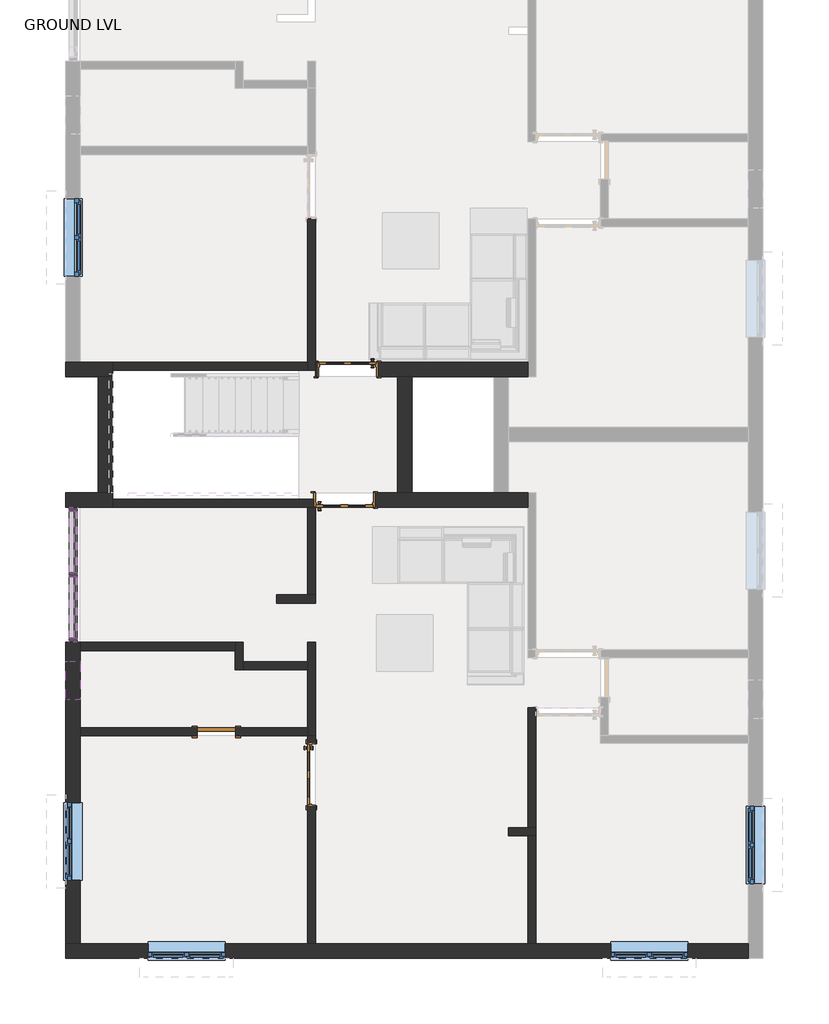
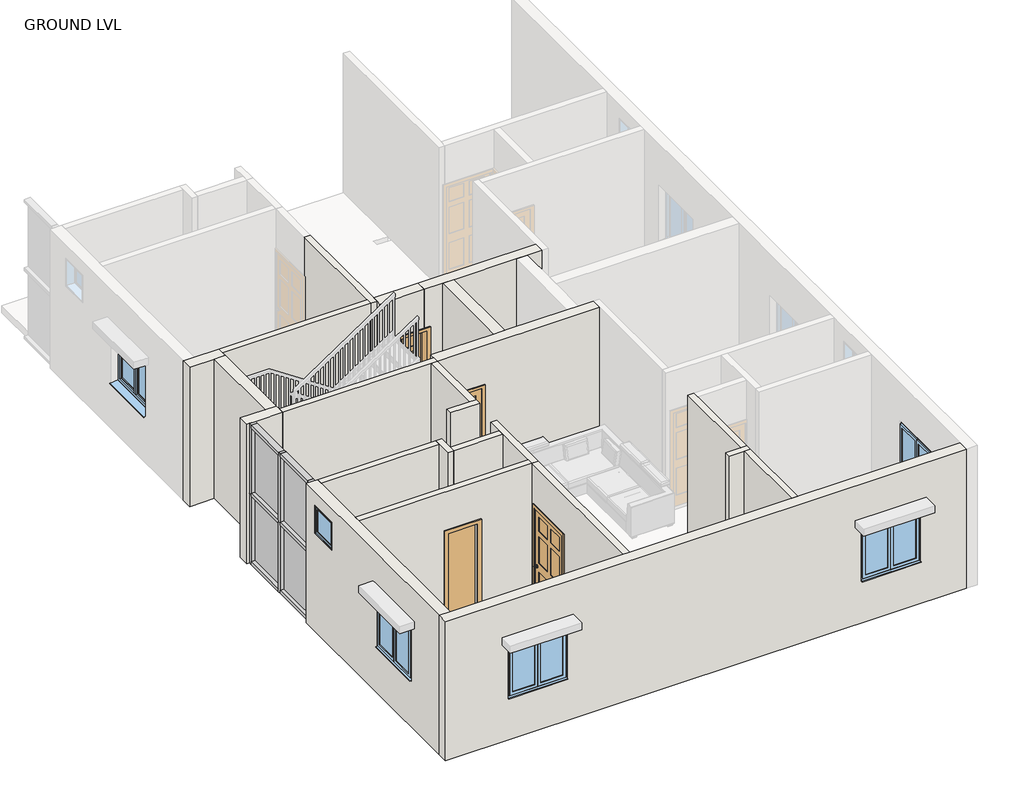
# One storey, part 1 of 4: 23 walls, 12 members, 6 windows, 4 doors, 4 plates.
"""IFC4 building model written with IfcOpenShell, lengths in millimetres."""

from ifc_helpers import new_model, si_unit, frame, origin, place, context, project, spatial, polyline, outline, extrude, faceted_brep, transform, mapped, element, save
from components import door_6a452240, door_interior_single_6_panel_wood_interior_door_3_x_7_c5239341, single_flush_flush_door_2_x_7_931cabab, member_801a2072, member_82905deb, member_88aa5c81, member_4491d118, system_panel_glazed_a8655be6, window_80340324, w2_windows_4_x_4_9dec5fc7

model = new_model("IFC4")

# Units and contexts
model_context = context("Model", 3, world=origin())
ifc_project = project(units=[si_unit("LENGTHUNIT", "METRE", prefix="MILLI")], contexts=[model_context])

# Site, building, storey
site = spatial("IfcSite", under=ifc_project)
building = spatial("IfcBuilding", under=site)
storey = spatial("IfcBuildingStorey", under=building, Name="GROUND LVL", Elevation=3048.0)

# Doors
placement = place(None, origin())
door_shape = door_6a452240(model_context)
element("IfcDoor", 1, ObjectType="Door-Interior-Single-6_Panel-Wood : interior door 3' 4\" x 7'", at=placement, inside=storey, context=model_context, shape_type="MappedRepresentation", body=[
    mapped(door_shape, transform((-2560.6762202, -343.1690997, 3048.0), x_axis=(0.0, -1.0, 0.0), y_axis=(1.0, 0.0, 0.0), z_axis=(0.0, 0.0, 1.0))),
])
door_interior_single_6_panel_wood_interior_door_3_x_7_shape = door_interior_single_6_panel_wood_interior_door_3_x_7_c5239341(model_context)
element("IfcDoor", 2, ObjectType="Door-Interior-Single-6_Panel-Wood : interior door 3' x 7'", at=placement, inside=storey, context=model_context, shape_type="MappedRepresentation", body=[
    mapped(door_interior_single_6_panel_wood_interior_door_3_x_7_shape, transform((-1986.0012202, 6048.1059003, 3048.0), x_axis=(-1.0, 0.0, 0.0), y_axis=(0.0, -1.0, 0.0), z_axis=(0.0, 0.0, 1.0))),
])
element("IfcDoor", 3, ObjectType="Door-Interior-Single-6_Panel-Wood : interior door 3' x 7'", at=placement, inside=storey, context=model_context, shape_type="MappedRepresentation", body=[
    mapped(door_interior_single_6_panel_wood_interior_door_3_x_7_shape, transform((-2036.8012202, 3984.3559003, 3048.0), x_axis=(1.0, 0.0, 0.0), y_axis=(0.0, 1.0, 0.0), z_axis=(0.0, 0.0, 1.0))),
])
single_flush_flush_door_2_x_7_shape = single_flush_flush_door_2_x_7_931cabab(model_context)
element("IfcDoor", 4, ObjectType="Single-Flush : flush door 2' x 7'", at=placement, inside=storey, context=model_context, shape_type="MappedRepresentation", body=[
    mapped(single_flush_flush_door_2_x_7_shape, transform((-4056.1012202, 329.9309003, 3048.0), x_axis=(-1.0, 0.0, 0.0), y_axis=(0.0, -1.0, 0.0), z_axis=(0.0, 0.0, 1.0))),
])

# Members
member_shape = member_801a2072(model_context)
element("IfcMember", 5, ObjectType="Rectangular Mullion : 2.5\" x 5\" rectangular", at=placement, inside=storey, context=model_context, shape_type="MappedRepresentation", body=[
    mapped(member_shape, transform((-6318.2887202, 1803.1309003, 6096.0), x_axis=(0.0, 0.0, 1.0), y_axis=(-1.0, 0.0, 0.0), z_axis=(0.0, -1.0, 0.0))),
])
element("IfcMember", 6, ObjectType="Rectangular Mullion : 2.5\" x 5\" rectangular", at=placement, inside=storey, context=model_context, shape_type="MappedRepresentation", body=[
    mapped(member_shape, transform((-6318.2887202, 2838.1809003, 6096.0), x_axis=(0.0, 0.0, 1.0), y_axis=(-1.0, 0.0, 0.0), z_axis=(0.0, -1.0, 0.0))),
])
element("IfcMember", 7, ObjectType="Rectangular Mullion : 2.5\" x 5\" rectangular", at=placement, inside=storey, context=model_context, shape_type="MappedRepresentation", body=[
    mapped(member_shape, transform((-6318.2887202, 3809.7309003, 3048.0), x_axis=(0.0, 0.0, -1.0), y_axis=(-1.0, 0.0, 0.0), z_axis=(0.0, 1.0, 0.0))),
])
element("IfcMember", 8, ObjectType="Rectangular Mullion : 2.5\" x 5\" rectangular", at=placement, inside=storey, context=model_context, shape_type="MappedRepresentation", body=[
    mapped(member_shape, transform((-6318.2887202, 2774.6809003, 3048.0), x_axis=(0.0, 0.0, -1.0), y_axis=(-1.0, 0.0, 0.0), z_axis=(0.0, 1.0, 0.0))),
])
member_2_shape = member_82905deb(model_context)
element("IfcMember", 9, ObjectType="Rectangular Mullion : 2.5\" x 5\" rectangular", at=placement, inside=storey, context=model_context, shape_type="MappedRepresentation", body=[
    mapped(member_2_shape, transform((-6318.2887202, 2806.4309003, 3048.0), x_axis=(0.0, -1.0, 0.0), y_axis=(-1.0, 0.0, 0.0), z_axis=(0.0, 0.0, -1.0))),
])
member_3_shape = member_88aa5c81(model_context)
element("IfcMember", 10, ObjectType="Rectangular Mullion : 2.5\" x 5\" rectangular", at=placement, inside=storey, context=model_context, shape_type="MappedRepresentation", body=[
    mapped(member_3_shape, transform((-6318.2887202, 2838.1809003, 4572.0), x_axis=(0.0, 0.0, 1.0), y_axis=(-1.0, 0.0, 0.0), z_axis=(0.0, -1.0, 0.0))),
])
element("IfcMember", 11, ObjectType="Rectangular Mullion : 2.5\" x 5\" rectangular", at=placement, inside=storey, context=model_context, shape_type="MappedRepresentation", body=[
    mapped(member_3_shape, transform((-6318.2887202, 1803.1309003, 4572.0), x_axis=(0.0, 0.0, 1.0), y_axis=(-1.0, 0.0, 0.0), z_axis=(0.0, -1.0, 0.0))),
])
element("IfcMember", 12, ObjectType="Rectangular Mullion : 2.5\" x 5\" rectangular", at=placement, inside=storey, context=model_context, shape_type="MappedRepresentation", body=[
    mapped(member_2_shape, transform((-6318.2887202, 2806.4309003, 4572.0), x_axis=(0.0, -1.0, 0.0), y_axis=(-1.0, 0.0, 0.0), z_axis=(0.0, 0.0, -1.0))),
])
member_4_shape = member_4491d118(model_context)
element("IfcMember", 13, ObjectType="Rectangular Mullion : 2.5\" x 5\" rectangular", at=placement, inside=storey, context=model_context, shape_type="MappedRepresentation", body=[
    mapped(member_4_shape, transform((-6318.2887202, 1739.6309003, 3048.0), x_axis=(0.0, -1.0, 0.0), y_axis=(-1.0, 0.0, 0.0), z_axis=(0.0, 0.0, -1.0))),
])
element("IfcMember", 14, ObjectType="Rectangular Mullion : 2.5\" x 5\" rectangular", at=placement, inside=storey, context=model_context, shape_type="MappedRepresentation", body=[
    mapped(member_4_shape, transform((-6318.2887202, 3873.2309003, 6096.0), x_axis=(0.0, 1.0, 0.0), y_axis=(-1.0, 0.0, 0.0), z_axis=(0.0, 0.0, 1.0))),
])
element("IfcMember", 15, ObjectType="Rectangular Mullion : 2.5\" x 5\" rectangular", at=placement, inside=storey, context=model_context, shape_type="MappedRepresentation", body=[
    mapped(member_4_shape, transform((-6318.2887202, 1739.6309003, 4572.0), x_axis=(0.0, -1.0, 0.0), y_axis=(-1.0, 0.0, 0.0), z_axis=(0.0, 0.0, -1.0))),
])
element("IfcMember", 16, ObjectType="Rectangular Mullion : 2.5\" x 5\" rectangular", at=placement, inside=storey, context=model_context, shape_type="MappedRepresentation", body=[
    mapped(member_4_shape, transform((-6318.2887202, 3873.2309003, 4572.0), x_axis=(0.0, 1.0, 0.0), y_axis=(-1.0, 0.0, 0.0), z_axis=(0.0, 0.0, 1.0))),
])

# Plates
system_panel_glazed_shape = system_panel_glazed_a8655be6(model_context)
element("IfcPlate", 17, ObjectType="System Panel : Glazed", at=placement, inside=storey, context=model_context, shape_type="MappedRepresentation", body=[
    mapped(system_panel_glazed_shape, transform((-6318.2887202, 3323.9559003, 3111.5), x_axis=(0.0, -1.0, 0.0), y_axis=(1.0, 0.0, 0.0), z_axis=(0.0, 0.0, 1.0))),
])
element("IfcPlate", 18, ObjectType="System Panel : Glazed", at=placement, inside=storey, context=model_context, shape_type="MappedRepresentation", body=[
    mapped(system_panel_glazed_shape, transform((-6318.2887202, 2288.9059003, 3111.5), x_axis=(0.0, -1.0, 0.0), y_axis=(1.0, 0.0, 0.0), z_axis=(0.0, 0.0, 1.0))),
])
element("IfcPlate", 19, ObjectType="System Panel : Glazed", at=placement, inside=storey, context=model_context, shape_type="MappedRepresentation", body=[
    mapped(system_panel_glazed_shape, transform((-6318.2887202, 3323.9559003, 4603.75), x_axis=(0.0, -1.0, 0.0), y_axis=(1.0, 0.0, 0.0), z_axis=(0.0, 0.0, 1.0))),
])
element("IfcPlate", 20, ObjectType="System Panel : Glazed", at=placement, inside=storey, context=model_context, shape_type="MappedRepresentation", body=[
    mapped(system_panel_glazed_shape, transform((-6318.2887202, 2288.9059003, 4603.75), x_axis=(0.0, -1.0, 0.0), y_axis=(1.0, 0.0, 0.0), z_axis=(0.0, 0.0, 1.0))),
])

# Walls
element("IfcWall", 21, ObjectType="OUTER WALL 9\"", at=placement, inside=storey, context=model_context, shape_type="Brep", body=[
    faceted_brep([(4338.5987798, -3010.1690997, 3048.0), (985.7987798, -3010.1690997, 3048.0), (858.7987798, -3010.1690997, 3048.0), (-2494.0012202, -3010.1690997, 3048.0), (-2621.0012202, -3010.1690997, 3048.0), (-6203.9887202, -3010.1690997, 3048.0), (-6432.5887202, -3010.1690997, 3048.0), (-6432.5887202, -3010.1690997, 6096.0), (-6203.9887202, -3010.1690997, 6096.0), (-2621.0012202, -3010.1690997, 6096.0), (-2494.0012202, -3010.1690997, 6096.0), (858.7987798, -3010.1690997, 6096.0), (985.7987798, -3010.1690997, 6096.0), (4338.5987798, -3010.1690997, 6096.0), (-5137.1887202, -3010.1690997, 3962.4), (-3917.9887202, -3010.1690997, 3962.4), (-3917.9887202, -3010.1690997, 5181.6), (-5137.1887202, -3010.1690997, 5181.6), (2166.8987798, -3010.1690997, 3962.4), (3386.0987798, -3010.1690997, 3962.4), (3386.0987798, -3010.1690997, 5181.6), (2166.8987798, -3010.1690997, 5181.6), (4338.5987798, -3238.7690997, 3048.0), (4338.5987798, -3238.7690997, 6096.0), (-6432.5887202, -3238.7690997, 6096.0), (-6432.5887202, -3238.7690997, 3048.0), (-5137.1887202, -3238.7690997, 3962.4), (-5137.1887202, -3238.7690997, 5181.6), (-3917.9887202, -3238.7690997, 5181.6), (-3917.9887202, -3238.7690997, 3962.4), (2166.8987798, -3238.7690997, 3962.4), (2166.8987798, -3238.7690997, 5181.6), (3386.0987798, -3238.7690997, 5181.6), (3386.0987798, -3238.7690997, 3962.4)], [[[0, 1, 2, 3, 4, 5, 6, 7, 8, 9, 10, 11, 12, 13], [14, 15, 16, 17], [18, 19, 20, 21]], [[22, 23, 24, 25], [26, 27, 28, 29], [30, 31, 32, 33]], [[6, 5, 4, 3, 2, 1, 0, 22, 25]], [[13, 12, 11, 10, 9, 8, 7, 24, 23]], [[0, 13, 23, 22]], [[7, 6, 25, 24]], [[27, 26, 14, 17]], [[28, 27, 17, 16]], [[29, 28, 16, 15]], [[26, 29, 15, 14]], [[31, 30, 18, 21]], [[32, 31, 21, 20]], [[33, 32, 20, 19]], [[30, 33, 19, 18]]]),
])
element("IfcWall", 22, ObjectType="OUTER WALL 9\"", at=placement, inside=storey, context=model_context, shape_type="Brep", body=[
    faceted_brep([(-6203.9887202, -3010.1690997, 6096.0), (-6203.9887202, -3010.1690997, 3048.0), (-6203.9887202, 266.4309003, 3048.0), (-6203.9887202, 393.4309003, 3048.0), (-6203.9887202, 1612.6309003, 3048.0), (-6203.9887202, 1739.6309003, 3048.0), (-6203.9887202, 1739.6309003, 6096.0), (-6203.9887202, 1612.6309003, 6096.0), (-6203.9887202, 393.4309003, 6096.0), (-6203.9887202, 266.4309003, 6096.0), (-6203.9887202, 1447.5309003, 5791.2), (-6203.9887202, 1447.5309003, 5181.6), (-6203.9887202, 837.9309003, 5181.6), (-6203.9887202, 837.9309003, 5791.2), (-6203.9887202, -787.6690997, 4048.0), (-6203.9887202, -2006.8690997, 4048.0), (-6203.9887202, -2006.8690997, 5267.2), (-6203.9887202, -787.6690997, 5267.2), (-6432.5887202, -3010.1690997, 3048.0), (-6432.5887202, -3010.1690997, 6096.0), (-6432.5887202, 1739.6309003, 6096.0), (-6432.5887202, 1739.6309003, 3048.0), (-6432.5887202, 1447.5309003, 5181.6), (-6432.5887202, 1447.5309003, 5791.2), (-6432.5887202, 837.9309003, 5791.2), (-6432.5887202, 837.9309003, 5181.6), (-6432.5887202, -787.6690997, 4048.0), (-6432.5887202, -787.6690997, 5267.2), (-6432.5887202, -2006.8690997, 5267.2), (-6432.5887202, -2006.8690997, 4048.0)], [[[0, 1, 2, 3, 4, 5, 6, 7, 8, 9], [10, 11, 12, 13], [14, 15, 16, 17]], [[18, 19, 20, 21], [22, 23, 24, 25], [26, 27, 28, 29]], [[1, 18, 21, 5, 4, 3, 2]], [[19, 0, 9, 8, 7, 6, 20]], [[1, 0, 19, 18]], [[10, 23, 22, 11]], [[11, 22, 25, 12]], [[24, 13, 12, 25]], [[23, 10, 13, 24]], [[6, 5, 21, 20]], [[27, 26, 14, 17]], [[28, 27, 17, 16]], [[29, 28, 16, 15]], [[26, 29, 15, 14]]]),
])
element("IfcWall", 23, ObjectType="OUTER WALL 9\"", at=placement, inside=storey, context=model_context, shape_type="Brep", body=[
    faceted_brep([(-6432.5887202, 3873.2309003, 3048.0), (-6203.9887202, 3873.2309003, 3048.0), (-5694.4012202, 3873.2309003, 3048.0), (-5694.4012202, 3873.2309003, 6096.0), (-6203.9887202, 3873.2309003, 6096.0), (-6432.5887202, 3873.2309003, 6096.0), (-6432.5887202, 4101.8309003, 3048.0), (-6432.5887202, 4101.8309003, 6096.0), (-5923.0012202, 4101.8309003, 6096.0), (-5694.4012202, 4101.8309003, 6096.0), (-5694.4012202, 4101.8309003, 3048.0), (-5923.0012202, 4101.8309003, 3048.0), (-5694.4012202, 4000.2309003, 3048.0), (-5694.4012202, 4000.2309003, 6096.0)], [[[0, 1, 2, 3, 4, 5]], [[6, 7, 8, 9, 10, 11]], [[2, 1, 0, 6, 11, 10, 12]], [[5, 4, 3, 13, 9, 8, 7]], [[0, 5, 7, 6]], [[3, 2, 12, 10, 9, 13]]]),
])
element("IfcWall", 24, ObjectType="OUTER WALL 9\"", at=placement, inside=storey, context=model_context, shape_type="SweptSolid", body=[
    extrude(outline(polyline([(-5694.4012202, 5930.6309003), (-5694.4012202, 4101.8309003), (-5923.0012202, 4101.8309003), (-5923.0012202, 5930.6309003), (-5694.4012202, 5930.6309003)])), frame((0.0, 0.0, 3048.0), z_axis=(0.0, 0.0, 1.0), x_axis=(1.0, 0.0, 0.0)), (0.0, 0.0, 1.0), 3048.0),
])
element("IfcWall", 25, ObjectType="OUTER WALL 9\"", at=placement, inside=storey, context=model_context, shape_type="Brep", body=[
    faceted_brep([(-5694.4012202, 6159.2309003, 3048.0), (-6202.4012202, 6159.2309003, 3048.0), (-6431.0012202, 6159.2309003, 3048.0), (-6431.0012202, 6159.2309003, 6096.0), (-6202.4012202, 6159.2309003, 6096.0), (-5694.4012202, 6159.2309003, 6096.0), (-5694.4012202, 5930.6309003, 3048.0), (-5694.4012202, 5930.6309003, 6096.0), (-5923.0012202, 5930.6309003, 6096.0), (-6431.0012202, 5930.6309003, 6096.0), (-6431.0012202, 5930.6309003, 3048.0), (-5923.0012202, 5930.6309003, 3048.0), (-5694.4012202, 6032.2309003, 3048.0), (-5694.4012202, 6032.2309003, 6096.0)], [[[0, 1, 2, 3, 4, 5]], [[6, 7, 8, 9, 10, 11]], [[2, 1, 0, 12, 6, 11, 10]], [[5, 4, 3, 9, 8, 7, 13]], [[0, 5, 13, 7, 6, 12]], [[3, 2, 10, 9]]]),
])
element("IfcWall", 26, ObjectType="OUTER WALL 9\"", at=placement, inside=storey, context=model_context, shape_type="Brep", body=[
    faceted_brep([(-2494.0012202, 4101.8309003, 6096.0), (-1198.6012202, 4101.8309003, 6096.0), (-970.0012202, 4101.8309003, 6096.0), (325.3987798, 4101.8309003, 6096.0), (553.9987798, 4101.8309003, 6096.0), (858.7987798, 4101.8309003, 6096.0), (858.7987798, 4101.8309003, 3048.0), (553.9987798, 4101.8309003, 3048.0), (325.3987798, 4101.8309003, 3048.0), (-970.0012202, 4101.8309003, 3048.0), (-1198.6012202, 4101.8309003, 3048.0), (-1554.2012202, 4101.8309003, 3048.0), (-1554.2012202, 4101.8309003, 5207.0), (-2494.0012202, 4101.8309003, 5207.0), (858.7987798, 3873.2309003, 6096.0), (-2494.0012202, 3873.2309003, 6096.0), (-2494.0012202, 3873.2309003, 5207.0), (-1554.2012202, 3873.2309003, 5207.0), (-1554.2012202, 3873.2309003, 3048.0), (858.7987798, 3873.2309003, 3048.0), (-2494.0012202, 4000.2309003, 6096.0), (-2494.0012202, 4000.2309003, 5207.0)], [[[0, 1, 2, 3, 4, 5, 6, 7, 8, 9, 10, 11, 12, 13]], [[14, 15, 16, 17, 18, 19]], [[6, 19, 18, 11, 10, 9, 8, 7]], [[5, 4, 3, 2, 1, 0, 20, 15, 14]], [[15, 20, 0, 13, 21, 16]], [[6, 5, 14, 19]], [[17, 12, 11, 18]], [[12, 17, 16, 21, 13]]]),
])
element("IfcWall", 27, ObjectType="OUTER WALL 9\"", at=placement, inside=storey, context=model_context, shape_type="SweptSolid", body=[
    extrude(outline(polyline([(-970.0012202, 5930.6309003), (-970.0012202, 4101.8309003), (-1198.6012202, 4101.8309003), (-1198.6012202, 5930.6309003), (-970.0012202, 5930.6309003)])), frame((0.0, 0.0, 3048.0), z_axis=(0.0, 0.0, 1.0), x_axis=(1.0, 0.0, 0.0)), (0.0, 0.0, 1.0), 3048.0),
])
element("IfcWall", 28, ObjectType="OUTER WALL 9\"", at=placement, inside=storey, context=model_context, shape_type="Brep", body=[
    faceted_brep([(858.7987798, 5930.6309003, 6096.0), (553.9987798, 5930.6309003, 6096.0), (325.3987798, 5930.6309003, 6096.0), (-970.0012202, 5930.6309003, 6096.0), (-1198.6012202, 5930.6309003, 6096.0), (-1579.6012202, 5930.6309003, 6096.0), (-1579.6012202, 5930.6309003, 5207.0), (-1503.4012202, 5930.6309003, 5207.0), (-1503.4012202, 5930.6309003, 3048.0), (-1198.6012202, 5930.6309003, 3048.0), (-970.0012202, 5930.6309003, 3048.0), (325.3987798, 5930.6309003, 3048.0), (553.9987798, 5930.6309003, 3048.0), (858.7987798, 5930.6309003, 3048.0), (-1579.6012202, 6159.2309003, 6096.0), (858.7987798, 6159.2309003, 6096.0), (858.7987798, 6159.2309003, 3048.0), (-1503.4012202, 6159.2309003, 3048.0), (-1503.4012202, 6159.2309003, 5207.0), (-1579.6012202, 6159.2309003, 5207.0)], [[[0, 1, 2, 3, 4, 5, 6, 7, 8, 9, 10, 11, 12, 13]], [[14, 15, 16, 17, 18, 19]], [[16, 13, 12, 11, 10, 9, 8, 17]], [[5, 4, 3, 2, 1, 0, 15, 14]], [[5, 14, 19, 6]], [[0, 13, 16, 15]], [[18, 7, 6, 19]], [[7, 18, 17, 8]]]),
])
element("IfcWall", 29, ObjectType="OUTER WALL 9\"", at=placement, inside=storey, context=model_context, shape_type="Brep", body=[
    faceted_brep([(-2494.0012202, 6159.2309003, 6096.0), (-1579.6012202, 6159.2309003, 6096.0), (-1579.6012202, 6159.2309003, 5207.0), (-2468.6012202, 6159.2309003, 5207.0), (-2468.6012202, 6159.2309003, 3048.0), (-2494.0012202, 6159.2309003, 3048.0), (-1579.6012202, 5930.6309003, 6096.0), (-2494.0012202, 5930.6309003, 6096.0), (-2494.0012202, 5930.6309003, 3048.0), (-2468.6012202, 5930.6309003, 3048.0), (-2468.6012202, 5930.6309003, 5207.0), (-1579.6012202, 5930.6309003, 5207.0), (-2494.0012202, 6032.2309003, 3048.0), (-2494.0012202, 6032.2309003, 6096.0)], [[[0, 1, 2, 3, 4, 5]], [[6, 7, 8, 9, 10, 11]], [[8, 12, 5, 4, 9]], [[1, 0, 13, 7, 6]], [[1, 6, 11, 2]], [[0, 5, 12, 8, 7, 13]], [[3, 10, 9, 4]], [[10, 3, 2, 11]]]),
])
element("IfcWall", 30, ObjectType="inner wall 5\"", at=placement, inside=storey, context=model_context, shape_type="Brep", body=[
    faceted_brep([(-2621.0012202, 8419.8309003, 3048.0), (-2621.0012202, 6159.2309003, 3048.0), (-2621.0012202, 6032.2309003, 3048.0), (-2621.0012202, 6032.2309003, 6096.0), (-2621.0012202, 6159.2309003, 6096.0), (-2621.0012202, 8419.8309003, 6096.0), (-2621.0012202, 8419.8309003, 5207.0), (-2494.0012202, 8419.8309003, 3048.0), (-2494.0012202, 8419.8309003, 5207.0), (-2494.0012202, 8419.8309003, 6096.0), (-2494.0012202, 6159.2309003, 6096.0), (-2494.0012202, 6032.2309003, 6096.0), (-2494.0012202, 6032.2309003, 3048.0), (-2494.0012202, 6159.2309003, 3048.0)], [[[0, 1, 2, 3, 4, 5, 6]], [[7, 8, 9, 10, 11, 12, 13]], [[2, 1, 0, 7, 13, 12]], [[5, 4, 3, 11, 10, 9]], [[0, 6, 5, 9, 8, 7]], [[3, 2, 12, 11]]]),
])
element("IfcWall", 31, ObjectType="inner wall 5\"", at=placement, inside=storey, context=model_context, shape_type="SweptSolid", body=[
    extrude(outline(polyline([(-2621.0012202, 6032.2309003), (-5694.4012202, 6032.2309003), (-5694.4012202, 6159.2309003), (-2621.0012202, 6159.2309003), (-2621.0012202, 6032.2309003)])), frame((0.0, 0.0, 3048.0), z_axis=(0.0, 0.0, 1.0), x_axis=(1.0, 0.0, 0.0)), (0.0, 0.0, 1.0), 3048.0),
])
element("IfcWall", 32, ObjectType="inner wall 5\"", at=placement, inside=storey, context=model_context, shape_type="Brep", body=[
    faceted_brep([(-2494.0012202, 3873.2309003, 6096.0), (-2621.0012202, 3873.2309003, 6096.0), (-5694.4012202, 3873.2309003, 6096.0), (-5694.4012202, 3873.2309003, 3048.0), (-2621.0012202, 3873.2309003, 3048.0), (-2519.4012202, 3873.2309003, 3048.0), (-2519.4012202, 3873.2309003, 5207.0), (-2494.0012202, 3873.2309003, 5207.0), (-5694.4012202, 4000.2309003, 6096.0), (-2494.0012202, 4000.2309003, 6096.0), (-2494.0012202, 4000.2309003, 5207.0), (-2519.4012202, 4000.2309003, 5207.0), (-2519.4012202, 4000.2309003, 3048.0), (-5694.4012202, 4000.2309003, 3048.0)], [[[0, 1, 2, 3, 4, 5, 6, 7]], [[8, 9, 10, 11, 12, 13]], [[3, 13, 12, 5, 4]], [[2, 1, 0, 9, 8]], [[3, 2, 8, 13]], [[9, 0, 7, 10]], [[6, 11, 10, 7]], [[11, 6, 5, 12]]]),
])
element("IfcWall", 33, ObjectType="inner wall 5\"", at=placement, inside=storey, context=model_context, shape_type="Brep", body=[
    faceted_brep([(-3103.6012202, 2361.9309003, 3048.0), (-2494.0012202, 2361.9309003, 3048.0), (-2494.0012202, 2361.9309003, 6096.0), (-3103.6012202, 2361.9309003, 6096.0), (-3103.6012202, 2488.9309003, 3048.0), (-3103.6012202, 2488.9309003, 6096.0), (-2621.0012202, 2488.9309003, 6096.0), (-2494.0012202, 2488.9309003, 6096.0), (-2494.0012202, 2488.9309003, 3048.0), (-2621.0012202, 2488.9309003, 3048.0)], [[[0, 1, 2, 3]], [[4, 5, 6, 7, 8, 9]], [[1, 0, 4, 9, 8]], [[3, 2, 7, 6, 5]], [[0, 3, 5, 4]], [[2, 1, 8, 7]]]),
])
element("IfcWall", 34, ObjectType="inner wall 5\"", at=placement, inside=storey, context=model_context, shape_type="Brep", body=[
    faceted_brep([(-2494.0012202, 2488.9309003, 3048.0), (-2494.0012202, 3873.2309003, 3048.0), (-2494.0012202, 3873.2309003, 5207.0), (-2494.0012202, 3873.2309003, 6096.0), (-2494.0012202, 2488.9309003, 6096.0), (-2621.0012202, 2488.9309003, 3048.0), (-2621.0012202, 2488.9309003, 6096.0), (-2621.0012202, 3873.2309003, 6096.0), (-2621.0012202, 3873.2309003, 3048.0), (-2519.4012202, 3873.2309003, 3048.0)], [[[0, 1, 2, 3, 4]], [[5, 6, 7, 8]], [[1, 0, 5, 8, 9]], [[4, 3, 7, 6]], [[0, 4, 6, 5]], [[3, 2, 1, 9, 8, 7]]]),
])
element("IfcWall", 35, ObjectType="inner wall 5\"", at=placement, inside=storey, context=model_context, shape_type="SweptSolid", body=[
    extrude(outline(polyline([(-3764.0012202, 1612.6309003), (-6203.9887202, 1612.6309003), (-6203.9887202, 1739.6309003), (-3764.0012202, 1739.6309003), (-3764.0012202, 1612.6309003)])), frame((0.0, 0.0, 3048.0), z_axis=(0.0, 0.0, 1.0), x_axis=(1.0, 0.0, 0.0)), (0.0, 0.0, 1.0), 3048.0),
])
element("IfcWall", 36, ObjectType="inner wall 5\"", at=placement, inside=storey, context=model_context, shape_type="Brep", body=[
    faceted_brep([(-3764.0012202, 1739.6309003, 3048.0), (-3764.0012202, 1612.6309003, 3048.0), (-3764.0012202, 1307.8309003, 3048.0), (-3764.0012202, 1307.8309003, 6096.0), (-3764.0012202, 1612.6309003, 6096.0), (-3764.0012202, 1739.6309003, 6096.0), (-3637.0012202, 1739.6309003, 3048.0), (-3637.0012202, 1739.6309003, 6096.0), (-3637.0012202, 1434.8309003, 6096.0), (-3637.0012202, 1307.8309003, 6096.0), (-3637.0012202, 1307.8309003, 3048.0), (-3637.0012202, 1434.8309003, 3048.0)], [[[0, 1, 2, 3, 4, 5]], [[6, 7, 8, 9, 10, 11]], [[2, 1, 0, 6, 11, 10]], [[5, 4, 3, 9, 8, 7]], [[0, 5, 7, 6]], [[3, 2, 10, 9]]]),
])
element("IfcWall", 37, ObjectType="inner wall 5\"", at=placement, inside=storey, context=model_context, shape_type="SweptSolid", body=[
    extrude(outline(polyline([(-2621.0012202, 1307.8309003), (-3637.0012202, 1307.8309003), (-3637.0012202, 1434.8309003), (-2621.0012202, 1434.8309003), (-2621.0012202, 1307.8309003)])), frame((0.0, 0.0, 3048.0), z_axis=(0.0, 0.0, 1.0), x_axis=(1.0, 0.0, 0.0)), (0.0, 0.0, 1.0), 3048.0),
])
element("IfcWall", 38, ObjectType="inner wall 5\"", at=placement, inside=storey, context=model_context, shape_type="Brep", body=[
    faceted_brep([(-2621.0012202, 1739.6309003, 3048.0), (-2621.0012202, 1434.8309003, 3048.0), (-2621.0012202, 1307.8309003, 3048.0), (-2621.0012202, 393.4309003, 3048.0), (-2621.0012202, 266.4309003, 3048.0), (-2621.0012202, 266.4309003, 6096.0), (-2621.0012202, 393.4309003, 6096.0), (-2621.0012202, 1307.8309003, 6096.0), (-2621.0012202, 1434.8309003, 6096.0), (-2621.0012202, 1739.6309003, 6096.0), (-2494.0012202, 1739.6309003, 3048.0), (-2494.0012202, 1739.6309003, 6096.0), (-2494.0012202, 266.4309003, 6096.0), (-2494.0012202, 266.4309003, 3048.0)], [[[0, 1, 2, 3, 4, 5, 6, 7, 8, 9]], [[10, 11, 12, 13]], [[4, 3, 2, 1, 0, 10, 13]], [[9, 8, 7, 6, 5, 12, 11]], [[0, 9, 11, 10]], [[5, 4, 13, 12]]]),
])
element("IfcWall", 39, ObjectType="inner wall 5\"", at=placement, inside=storey, context=model_context, shape_type="SweptSolid", body=[
    extrude(outline(polyline([(3048.0, -6203.9887202), (3048.0, -4360.9012202), (5181.6, -4360.9012202), (5181.6, -3751.3012202), (3048.0, -3751.3012202), (3048.0, -2621.0012202), (6096.0, -2621.0012202), (6096.0, -6203.9887202), (3048.0, -6203.9887202)])), frame((0.0, 266.4309003, 0.0), z_axis=(0.0, 1.0, 0.0), x_axis=(0.0, 0.0, 1.0)), (0.0, 0.0, 1.0), 127.0),
])
element("IfcWall", 40, ObjectType="inner wall 5\"", at=placement, inside=storey, context=model_context, shape_type="SweptSolid", body=[
    extrude(outline(polyline([(-3010.1690997, 6096.0), (266.4309003, 6096.0), (266.4309003, 3048.0), (164.8309003, 3048.0), (164.8309003, 5207.0), (-851.1690997, 5207.0), (-851.1690997, 3048.0), (-3010.1690997, 3048.0), (-3010.1690997, 6096.0)])), frame((-2621.0012202, 0.0, 0.0), z_axis=(1.0, 0.0, 0.0), x_axis=(0.0, 1.0, 0.0)), (0.0, 0.0, 1.0), 127.0),
])
element("IfcWall", 41, ObjectType="inner wall 5\"", at=placement, inside=storey, context=model_context, shape_type="SweptSolid", body=[
    extrude(outline(polyline([(985.7987798, -1308.3690997), (985.7987798, -3010.1690997), (858.7987798, -3010.1690997), (858.7987798, -1308.3690997), (985.7987798, -1308.3690997)])), frame((0.0, 0.0, 3048.0), z_axis=(0.0, 0.0, 1.0), x_axis=(1.0, 0.0, 0.0)), (0.0, 0.0, 1.0), 3048.0),
])
element("IfcWall", 42, ObjectType="inner wall 5\"", at=placement, inside=storey, context=model_context, shape_type="Brep", body=[
    faceted_brep([(553.9987798, -1308.3690997, 3048.0), (985.7987798, -1308.3690997, 3048.0), (985.7987798, -1308.3690997, 6096.0), (553.9987798, -1308.3690997, 6096.0), (553.9987798, -1181.3690997, 3048.0), (553.9987798, -1181.3690997, 6096.0), (858.7987798, -1181.3690997, 6096.0), (985.7987798, -1181.3690997, 6096.0), (985.7987798, -1181.3690997, 3048.0), (858.7987798, -1181.3690997, 3048.0)], [[[0, 1, 2, 3]], [[4, 5, 6, 7, 8, 9]], [[1, 0, 4, 9, 8]], [[3, 2, 7, 6, 5]], [[0, 3, 5, 4]], [[2, 1, 8, 7]]]),
])
element("IfcWall", 43, ObjectType="inner wall 5\"", at=placement, inside=storey, context=model_context, shape_type="Brep", body=[
    faceted_brep([(985.7987798, -1181.3690997, 3048.0), (985.7987798, 710.9309003, 3048.0), (985.7987798, 710.9309003, 5207.0), (985.7987798, 710.9309003, 6096.0), (985.7987798, 583.9309003, 6096.0), (985.7987798, -1181.3690997, 6096.0), (858.7987798, -1181.3690997, 3048.0), (858.7987798, -1181.3690997, 6096.0), (858.7987798, 710.9309003, 6096.0), (858.7987798, 710.9309003, 3048.0)], [[[0, 1, 2, 3, 4, 5]], [[6, 7, 8, 9]], [[1, 0, 6, 9]], [[5, 4, 3, 8, 7]], [[0, 5, 7, 6]], [[3, 2, 1, 9, 8]]]),
])

# Windows
window_shape = window_80340324(model_context)
element("IfcWindow", 44, ObjectType="Fixed : 24\" x 24\"", at=placement, inside=storey, context=model_context, shape_type="MappedRepresentation", body=[
    mapped(window_shape, transform((-6318.2887202, 1180.8309003, 4267.2), x_axis=(0.0, 1.0, 0.0), y_axis=(-1.0, 0.0, 0.0), z_axis=(0.0, 0.0, 1.0))),
])
w2_windows_4_x_4_shape = w2_windows_4_x_4_9dec5fc7(model_context)
element("IfcWindow", 45, ObjectType="w2 : windows 4' x 4'", at=placement, inside=storey, context=model_context, shape_type="MappedRepresentation", body=[
    mapped(w2_windows_4_x_4_shape, transform((-4527.5887202, -3124.4690997, 2962.4), x_axis=(1.0, 0.0, 0.0), y_axis=(0.0, 1.0, 0.0), z_axis=(0.0, 0.0, 1.0))),
])
element("IfcWindow", 46, ObjectType="w2 : windows 4' x 4'", at=placement, inside=storey, context=model_context, shape_type="MappedRepresentation", body=[
    mapped(w2_windows_4_x_4_shape, transform((2776.4987798, -3124.4690997, 2962.4), x_axis=(1.0, 0.0, 0.0), y_axis=(0.0, 1.0, 0.0), z_axis=(0.0, 0.0, 1.0))),
])
element("IfcWindow", 47, ObjectType="w2 : windows 4' x 4'", at=placement, inside=storey, context=model_context, shape_type="MappedRepresentation", body=[
    mapped(w2_windows_4_x_4_shape, transform((-6316.7012202, 8127.7309003, 3048.0), x_axis=(0.0, 1.0, 0.0), y_axis=(-1.0, 0.0, 0.0), z_axis=(0.0, 0.0, 1.0))),
])
element("IfcWindow", 48, ObjectType="w2 : windows 4' x 4'", at=placement, inside=storey, context=model_context, shape_type="MappedRepresentation", body=[
    mapped(w2_windows_4_x_4_shape, transform((4452.8987798, -1454.4190997, 3048.0), x_axis=(0.0, -1.0, 0.0), y_axis=(1.0, 0.0, 0.0), z_axis=(0.0, 0.0, 1.0))),
])
element("IfcWindow", 49, ObjectType="w2 : windows 4' x 4'", at=placement, inside=storey, context=model_context, shape_type="MappedRepresentation", body=[
    mapped(w2_windows_4_x_4_shape, transform((-6318.2887202, -1397.2690997, 3048.0), x_axis=(0.0, -1.0, 0.0), y_axis=(1.0, 0.0, 0.0), z_axis=(0.0, 0.0, 1.0))),
])

save(model, "model.ifc")

# Revit data of these elements
# Type "Door-Interior-Single-6_Panel-Wood : interior door 3' 4\" x 7'"
#   Type Mark = "11"
#   Assembly Code = "C1020300"
#   Analytic Construction = "Wooden"
#   Top Rail = 0' - 4 11/16"
#   Top Panel = 1' - 0"
#   Thickness = 0' - 1 3/8"
#   Thermal Resistance (R) = 2.5876 (h·ft²·°F)/BTU
#   Swing Angle [instance default] = 90.00°
#   Stiles = 0' - 4 3/4"
#   Rough Width = 3' - 4"
#   Rough Height = 7' - 1"
#   Mullion = 0' - 4 1/2"
#   Lock Rail = 0' - 7 1/2"
#   Intermediate Rail = 0' - 4 1/2"
#   Height = 7' - 0"
#   Width = 3' - 2"
#   Heat Transfer Coefficient (U) = 0.3865 BTU/(h·ft²·°F)
#   Bottom Rail = 0' - 9 1/8"
#   Trim Material = Cherry
#   Panel Material = Cherry
#   Frame Material = Cherry
#   Door Handle Material = Aluminum
#   Visual Light Transmittance = 0
#   Solar Heat Gain Coefficient = 0
#   Wall Closure = (empty or 0)
#   Function = (empty or 0)
# Type "Door-Interior-Single-6_Panel-Wood : interior door 3' x 7'"
#   Type Mark = "13"
#   Assembly Code = "C1020300"
#   Analytic Construction = "Wooden"
#   Top Rail = 0' - 4 11/16"
#   Top Panel = 0' - 11"
#   Thickness = 0' - 1 3/8"
#   Thermal Resistance (R) = 2.5876 (h·ft²·°F)/BTU
#   Swing Angle [instance default] = 90.00°
#   Stiles = 0' - 4 3/4"
#   Rough Width = 3' - 2"
#   Rough Height = 7' - 1"
#   Mullion = 0' - 4 1/2"
#   Lock Rail = 0' - 7 1/2"
#   Intermediate Rail = 0' - 4 1/2"
#   Height = 7' - 0"
#   Width = 3' - 0"
#   Heat Transfer Coefficient (U) = 0.3865 BTU/(h·ft²·°F)
#   Bottom Rail = 0' - 9 1/8"
#   Trim Material = Cherry
#   Panel Material = Cherry
#   Frame Material = Cherry
#   Door Handle Material = Aluminum
#   Visual Light Transmittance = 0
#   Solar Heat Gain Coefficient = 0
#   Wall Closure = (empty or 0)
#   Function = (empty or 0)
# Type "Single-Flush : flush door 2' x 7'"
#   Type Mark = "12"
#   Construction Type Id = "MDOOR"
#   Assembly Code = "C1020"
#   Analytic Construction = "Metal"
#   Thickness = 0' - 2"
#   Heat Transfer Coefficient (U) = 0.651978 BTU/(h·ft²·°F)
#   Height = 7' - 0"
#   Trim Projection Ext = 0' - 1"
#   Trim Projection Int = 0' - 1"
#   Trim Width = 0' - 3"
#   Width = 2' - 0"
#   Define Thermal Properties by = 1
#   Door Material = Door - Panel
#   Frame Material = Door - Frame
#   Visual Light Transmittance = 0
#   Solar Heat Gain Coefficient = 0
#   Function = (empty or 0)
#   Wall Closure = (empty or 0)
# Type "Rectangular Mullion : 2.5\" x 5\" rectangular"
#   built-in parameter 1007304 = 0.416667 (stored number, unit not read)
#   built-in parameter 1007301 = 0.104167 (stored number, unit not read)
#   built-in parameter 1007300 = 0.104167 (stored number, unit not read)
# Type "System Panel : Glazed"
#   Construction Type Id = "GSP4R"
#   Analytic Construction = "1/8 in Pilkington single glazing"
#   Visual Light Transmittance = 0.9
#   Solar Heat Gain Coefficient = 0.86
#   Heat Transfer Coefficient (U) = 1.18115 BTU/(h·ft²·°F)
#   Define Thermal Properties by = 1
# Type "OUTER WALL 9\""
#   Assembly Code = "B2010"
#   Layers, outside or top first: 0' - 9" "ROSE COLOUR" (function 1)
# Type "inner wall 5\""
#   Assembly Code = "B2010"
#   Layers, outside or top first: 0' - 5" "ROSE COLOUR" (function 1)
# Type "Fixed : 24\" x 24\""
#   Type Mark = "3"
#   Construction Type Id = "GSP4R"
#   Assembly Code = "B2020100"
#   Analytic Construction = "1/8 in Pilkington single glazing"
#   Visual Light Transmittance = 0.9
#   Solar Heat Gain Coefficient = 0.78
#   Heat Transfer Coefficient (U) = 0.6496 BTU/(h·ft²·°F)
#   Height = 2' - 0"
#   Default Sill Height = 3' - 0"
#   Width = 2' - 0"
#   Window Inset = 0' - 0 3/4"
#   Define Thermal Properties by = 1
#   Define Thermal Properties by = 1
#   Glass Pane Material = Glass
#   Sash Material = Sash
#   Wall Closure = (empty or 0)
# Type "w2 : windows 4' x 4'"
#   Type Mark = "31"
#   Operation = "DoublePanelVertical"
#   Keynote = "16.05.01"
#   Analytic Construction = "<None>"
#   Rough Width = 4' - 0"
#   Rough Height = 4' - 0"
#   Rahmentiefe = 0' - 2.3622"
#   Rahmenhöhe unten = 0' - 3.14961"
#   Rahmehöhe oben = 0' - 3.14961"
#   Rahmenbreite = 0' - 2.3622"
#   Heat Transfer Coefficient (U) = 2.81836 BTU/(h·ft²·°F)
#   Height = 4' - 0"
#   Flügeltiefe = 0' - 2.3622"
#   Flügelbreite = 0' - 2.3622"
#   Einbautiefe (von außen) [instance default] = 0' - 5.51181"
#   Width = 4' - 0"
#   Kippflügel [instance default] = yes
#   Drehflügel im Grundriß darstellen [instance default] = no
#   Drehflügel [instance default] = yes
#   Define Thermal Properties by = 1
#   Rahmen [instance default] = none
#   Glas [instance default] = blue glass
#   Flügel [instance default] = WINDOW COLOUR WHITE
#   Fensterbank aussen [instance default] = WINDOW COLOUR WHITE
#   Fensterbank innen [instance default] = WINDOW COLOUR WHITE
#   Visual Light Transmittance = 0
#   Thermal Resistance (R) = 0
#   Solar Heat Gain Coefficient = 0
#   Wall Closure = (empty or 0)
# Element 1 (IfcDoor, "Door-Interior-Single-6_Panel-Wood : interior door 3' 4\" x 7'")
#   Swing Angle = 90.00°
#   Phase Created = New Construction
#   Materials on its faces: "Cherry", "Aluminum"
# Elements 2, 3 (IfcDoor, "Door-Interior-Single-6_Panel-Wood : interior door 3' x 7'")
#   Swing Angle = 90.00°
#   Phase Created = New Construction
#   Materials on its faces: "Cherry", "Aluminum"
# Element 4 (IfcDoor, "Single-Flush : flush door 2' x 7'")
#   Phase Created = New Construction
#   Materials on its faces: "Door - Frame", "Door - Panel"
# Elements 5, 6, 7, 8, 9, 10, 11, 12, 13, 14, 15, 16 (IfcMember, "Rectangular Mullion : 2.5\" x 5\" rectangular")
#   Phase Created = New Construction
#   Materials on its faces: "Aluminum"
# Elements 17, 18, 19, 20 (IfcPlate, "System Panel : Glazed")
#   Phase Created = New Construction
#   Materials on its faces: "Glass"
# Elements 21, 22, 23, 24, 25, 26, 27, 28, 29 (IfcWall, "OUTER WALL 9\"")
#   Top Offset = 0' - 0"
#   Base Offset = 0' - 0"
#   wall height = 10' - 0"
#   Phase Created = New Construction
#   Base Constraint = GROUND LVL
#   Top Constraint = 1 ST FLOOR
#   Materials on its faces: "ROSE COLOUR"
# Elements 30, 31, 32, 33, 34, 35, 36, 37, 38, 39, 40, 41, 42, 43 (IfcWall, "inner wall 5\"")
#   Top Offset = 0' - 0"
#   Base Offset = 0' - 0"
#   wall height = 10' - 0"
#   Phase Created = New Construction
#   Base Constraint = GROUND LVL
#   Top Constraint = 1 ST FLOOR
#   Materials on its faces: "ROSE COLOUR"
# Element 44 (IfcWindow, "Fixed : 24\" x 24\"")
#   Mark = "14"
#   Phase Created = New Construction
#   Materials on its faces: "Sash", "Glass"
# Element 45 (IfcWindow, "w2 : windows 4' x 4'")
#   Mark = "9"
#   Phase Created = New Construction
#   Materials on its faces: "WINDOW COLOUR WHITE", "blue glass"
# Element 46 (IfcWindow, "w2 : windows 4' x 4'")
#   Mark = "10"
#   Phase Created = New Construction
#   Materials on its faces: "WINDOW COLOUR WHITE", "blue glass"
# Element 47 (IfcWindow, "w2 : windows 4' x 4'")
#   Mark = "21"
#   Einbautiefe (von außen) = 0' - 5.51181"
#   Kippflügel = yes
#   Drehflügel im Grundriß darstellen = no
#   Drehflügel = yes
#   Rahmen = none
#   Glas = blue glass
#   Flügel = WINDOW COLOUR WHITE
#   Fensterbank innen = WINDOW COLOUR WHITE
#   Fensterbank aussen = WINDOW COLOUR WHITE
#   Phase Created = New Construction
#   Materials on its faces: "WINDOW COLOUR WHITE", "blue glass"
# Element 48 (IfcWindow, "w2 : windows 4' x 4'")
#   Mark = "22"
#   Einbautiefe (von außen) = 0' - 5.51181"
#   Kippflügel = yes
#   Drehflügel im Grundriß darstellen = no
#   Drehflügel = yes
#   Rahmen = none
#   Glas = blue glass
#   Flügel = WINDOW COLOUR WHITE
#   Fensterbank innen = WINDOW COLOUR WHITE
#   Fensterbank aussen = WINDOW COLOUR WHITE
#   Phase Created = New Construction
#   Materials on its faces: "WINDOW COLOUR WHITE", "blue glass"
# Element 49 (IfcWindow, "w2 : windows 4' x 4'")
#   Mark = "23"
#   Einbautiefe (von außen) = 0' - 5.51181"
#   Kippflügel = yes
#   Drehflügel im Grundriß darstellen = no
#   Drehflügel = yes
#   Rahmen = none
#   Glas = blue glass
#   Flügel = WINDOW COLOUR WHITE
#   Fensterbank innen = WINDOW COLOUR WHITE
#   Fensterbank aussen = WINDOW COLOUR WHITE
#   Phase Created = New Construction
#   Materials on its faces: "WINDOW COLOUR WHITE", "blue glass"
# Materials
#   "Cherry": class "Wood", colour RGB 226 177 128, transparency 0, Description = "Prunus Serotina", Cost = 0
#   "Aluminum": class "Metal", colour RGB 247 247 247, transparency 0, Description = "Aluminum 6061", Cost = 0
#   "Door - Panel": class "Wood", colour RGB 210 159 95, transparency 0, Cost = 0
#   "Door - Frame": colour RGB 118 70 51, transparency 0, Cost = 0
#   "ROSE COLOUR": class "Generic", colour RGB 120 120 120, transparency 0, Cost = 0
#   "Glass": class "Glass", colour RGB 0 128 192, transparency 0.75, Description = "Soda Lime Glass", Cost = 0
#   "Sash": class "Wood", colour RGB 224 178 126, transparency 0, Cost = 0
#   "blue glass": class "System", colour RGB 0 0 255, transparency 0.75, Cost = 0
#   "WINDOW COLOUR WHITE": class "Generic", colour RGB 120 120 120, transparency 0, Cost = 0
# Room at (3259.099, 9029.431) mm, phase "New Construction", upper level "GROUND LVL", upper offset 10' - 0", lower offset 0' - 0"
#   Number = ""
#   Name = "TOILET"
# Room at (-4437.101, 10172.431) mm, phase "New Construction", upper level "GROUND LVL", upper offset 10' - 0", lower offset 0' - 0"
#   Number = ""
#   Name = "TOILET"
# Room at (-4437.895, 1003.031) mm, phase "New Construction", upper level "GROUND LVL", upper offset 10' - 0", lower offset 0' - 0"
#   Number = ""
#   Name = "TOILET"
# Room at (-4437.895, -1397.269) mm, phase "New Construction", upper level "GROUND LVL", upper offset 10' - 0", lower offset 0' - 0"
#   Number = "5"
#   Name = "BEDROOM"
# Room at (-322.301, 5016.231) mm, phase "New Construction", upper level "GROUND LVL", upper offset 10' - 0", lower offset 0' - 0"
#   Number = "6"
#   Name = "LIFT"
# Room at (2446.299, 6686.281) mm, phase "New Construction", upper level "GROUND LVL", upper offset 10' - 0", lower offset 0' - 0"
#   Number = "7"
#   Name = "BEDROOM"
# Room at (2446.299, 3289.031) mm, phase "New Construction", upper level "GROUND LVL", upper offset 10' - 0", lower offset 0' - 0"
#   Number = "8"
#   Name = "BEDROOM"
# Room at (-4437.101, 7772.131) mm, phase "New Construction", upper level "GROUND LVL", upper offset 10' - 0", lower offset 0' - 0"
#   Number = "2"
#   Name = "BEDROOM"
# Room at (2687.599, 11429.731) mm, phase "New Construction", upper level "GROUND LVL", upper offset 10' - 0", lower offset 0' - 0"
#   Number = "1"
#   Name = "BED ROOM"
# Room at (-3446.501, 5016.231) mm, phase "New Construction", upper level "GROUND LVL", upper offset 10' - 0", lower offset 0' - 0"
#   Number = "10"
#   Name = "STAIRS"
# Room at (2687.599, -1238.519) mm, phase "New Construction", upper level "GROUND LVL", upper offset 10' - 0", lower offset 0' - 0"
#   Number = "11"
#   Name = "BEDROOM"
# Room at (3259.099, 888.731) mm, phase "New Construction", upper level "GROUND LVL", upper offset 10' - 0", lower offset 0' - 0"
#   Number = "12"
#   Name = "TOILET"
# Room at (-4437.101, 11848.831) mm, phase "New Construction", upper level "GROUND LVL", upper offset 10' - 0", lower offset 0' - 0"
#   Number = "ROOM"
#   Name = "KITCHEN"
# Room at (-246.101, 9600.931) mm, phase "New Construction", upper level "GROUND LVL", upper offset 10' - 0", lower offset 0' - 0"
#   Number = "14"
#   Name = "LIVING ROOM"
# Room at (-4437.895, 2679.431) mm, phase "New Construction", upper level "GROUND LVL", upper offset 10' - 0", lower offset 0' - 0"
#   Number = "15"
#   Name = "KITCHEN"
# Room at (-246.101, 431.531) mm, phase "New Construction", upper level "GROUND LVL", upper offset 10' - 0", lower offset 0' - 0"
#   Number = "16"
#   Name = "LIVING ROOM"
